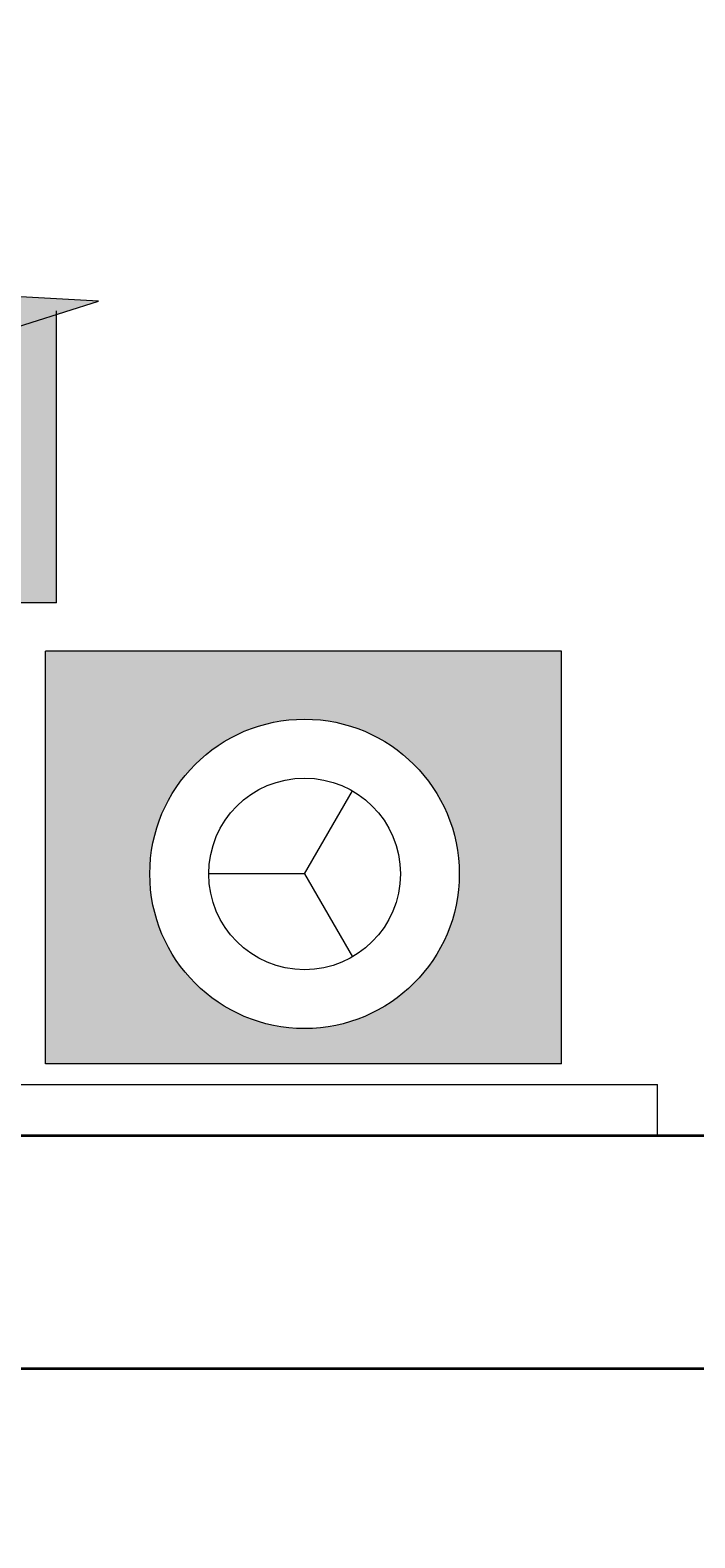
# Model space of a CAD drawing. Units: millimetres. Extents: x 27017497 to 27018854, y 7058029 to 7059154.
# Tile 76 of 91: x 27018436 to 27018462, y 7058126 to 7058185. Entities that reach past the tile are written whole.
import ezdxf

# ---------------------------------------------------------------- set-up
doc = ezdxf.new("R2010")
doc.units = ezdxf.units.MM
for name, color, linetype, lineweight in [('A-ANNO-DIMS', 2, 'Continuous', 18), ('A-FURN', 8, 'Continuous', 18), ('A-WALL', 7, 'Continuous', 35)]:
    doc.layers.add(name, color=color, linetype=linetype, lineweight=lineweight)
doc.layers.add('A-FURN-PATT', color=177, linetype='Continuous', lineweight=13, true_color=0x293189)
doc.styles.get("Standard").update_dxf_attribs({"font": 'arial.ttf'})
doc.dimstyles.get("Standard").update_dxf_attribs({"dimtxt": 0.18, "dimasz": 0.18, "dimexe": 0.18, "dimexo": 0.0625, "dimgap": 0.09, "dimtad": 0, "dimtih": 1, "dimtoh": 1, "dimdec": 4, "dimzin": 0, "dimdsep": 46, "dimtxsty": 'Standard', "dimcen": 0.09, "dimadec": 0, "dimazin": 0, "dimtfac": 1, "dimtdec": 4, "dimtofl": 0, "dimtmove": 0, "dimatfit": 3, "dimfxl": 1, "dimtolj": 1, "dimtzin": 0, "dimarcsym": 0})

# ---------------------------------------------------------------- blocks, each defined once
blk = doc.blocks.new('CAMMAT')
for p, q in [((1.2731, 0), (-1.2731, 0)), ((-1.2731, 0), (-1.2731, -0.05)), ((1.2731, -0.05), (-1.2731, -0.05)), ((-1.18, -0.07), (-1.18, -0.47)), ((-1.18, -0.07), (-0.68, -0.07)), ((-0.68, -0.07), (-0.68, -0.47)), ((-0.931, -0.2541), (-0.9775, -0.1737)), ((-0.931, -0.2541), (-0.9775, -0.3346)), ((-0.931, -0.2541), (-0.8381, -0.2541)), ((-1.18, -0.47), (-0.68, -0.47)), ((-0.6904, -0.5169), (-0.6904, -0.8)), ((-0.6904, -0.5169), (0.6826, -0.5169)), ((0.0535, -0.5623), (-0.7312, -0.8093))]:
    blk.add_line(p, q)
blk.add_lwpolyline([(-0.7312, -0.8093), (-0.5683, -0.8185), (-0.4451, -0.828), (-0.3552, -0.8406), (-0.2919, -0.8591), (-0.2489, -0.8862), (-0.2196, -0.9248), (-0.1975, -0.9777), (-0.1761, -1.0476)])
for radius in [0.15, 0.0929]:
    blk.add_circle((-0.931, -0.2541), radius)
blk = doc.blocks.new('*D47')
at = {"layer": 'A-ANNO-DIMS', "color": 0, "lineweight": -2, "transparency": 16777216}
for p, q in [((27017561.166, 7058294.35), (27017561.166, 7058028.6)), ((27018790.606, 7058294.35), (27018790.606, 7058028.6)), ((27017561.346, 7058028.78), (27018175.431, 7058028.78)), ((27018790.426, 7058028.78), (27018176.341, 7058028.78))]:
    blk.add_line(p, q, dxfattribs=at)
at = {"layer": 'A-ANNO-DIMS', "color": 0, "transparency": 16777216}
for points in [[(27017561.346, 7058028.81), (27017561.346, 7058028.75), (27017561.166, 7058028.78)], [(27018790.426, 7058028.81), (27018790.426, 7058028.75), (27018790.606, 7058028.78)]]:
    blk.add_solid(points, dxfattribs=at)
at = {"layer": 'Defpoints', "color": 0, "transparency": 16777216}
for p in [(27017561.166, 7058294.412), (27018790.606, 7058294.412), (27018790.606, 7058028.78)]:
    blk.add_point(p, dxfattribs=at)
at = {"layer": 'A-ANNO-DIMS', "color": 0, "transparency": 16777216, "insert": (27018175.886, 7058028.78), "char_height": 0.18, "attachment_point": 5}
blk.add_mtext('\\A1;1229.4', dxfattribs=at)
blk = doc.blocks.new('*D48')
at = {"layer": 'A-ANNO-DIMS', "color": 0, "lineweight": -2, "transparency": 16777216}
for p, q in [((27018463.498, 7058622.912), (27017497.536, 7058622.912)), ((27017497.716, 7058622.732), (27017497.716, 7058357.753)), ((27017497.716, 7058092.41), (27017497.716, 7058357.389)), ((27018555.129, 7058092.23), (27017497.536, 7058092.23))]:
    blk.add_line(p, q, dxfattribs=at)
at = {"layer": 'A-ANNO-DIMS', "color": 0, "transparency": 16777216}
for points in [[(27017497.686, 7058622.732), (27017497.746, 7058622.732), (27017497.716, 7058622.912)], [(27017497.686, 7058092.41), (27017497.746, 7058092.41), (27017497.716, 7058092.23)]]:
    blk.add_solid(points, dxfattribs=at)
at = {"layer": 'Defpoints', "color": 0, "transparency": 16777216}
for p in [(27018463.561, 7058622.912), (27017497.716, 7058092.23), (27018555.192, 7058092.23)]:
    blk.add_point(p, dxfattribs=at)
at = {"layer": 'A-ANNO-DIMS', "color": 0, "transparency": 16777216, "insert": (27017497.716, 7058357.571), "char_height": 0.18, "attachment_point": 5}
blk.add_mtext('\\A1;530.7', dxfattribs=at)

msp = doc.modelspace()

# ---------------------------------------------------------------- hatches: boundary and pattern name
at = {"layer": 'A-FURN-PATT'}
h = msp.add_hatch(color=256, dxfattribs=at)
h.dxf.hatch_style = 1
h.paths.add_polyline_path([(27018435.86, 7058218.784, 0.414214), (27018434.267, 7058220.377), (27018385.674, 7058220.377, 0.414214), (27018384.081, 7058218.784), (27018384.081, 7058174.59), (27018387.977, 7058174.891), (27018391.56, 7058175.393), (27018394.078, 7058176.128), (27018395.791, 7058177.21), (27018396.958, 7058178.748), (27018397.838, 7058180.854), (27018398.69, 7058183.639), (27018399.293, 7058180.835), (27018399.836, 7058178.594), (27018400.426, 7058176.691), (27018401.17, 7058174.899), (27018402.177, 7058172.991), (27018403.552, 7058170.741), (27018405.403, 7058167.922), (27018407.838, 7058164.308), (27018410.273, 7058167.922), (27018412.124, 7058170.741), (27018413.499, 7058172.991), (27018414.506, 7058174.899), (27018415.25, 7058176.691), (27018415.84, 7058178.594), (27018416.383, 7058180.835), (27018416.986, 7058183.639), (27018417.838, 7058180.854), (27018418.718, 7058178.748), (27018419.885, 7058177.21), (27018421.598, 7058176.128), (27018424.116, 7058175.393), (27018427.699, 7058174.891), (27018432.604, 7058174.513), (27018435.86, 7058174.329)])
h.paths.add_polyline_path([(27018439.093, 7058174.146), (27018432.604, 7058174.513), (27018427.699, 7058174.891), (27018424.116, 7058175.393), (27018421.598, 7058176.128), (27018419.885, 7058177.21), (27018418.718, 7058178.748), (27018417.838, 7058180.854), (27018416.986, 7058183.639), (27018416.383, 7058180.835), (27018415.84, 7058178.594), (27018415.25, 7058176.691), (27018414.506, 7058174.899), (27018413.499, 7058172.991), (27018412.124, 7058170.741), (27018410.273, 7058167.922), (27018407.838, 7058164.308)])
h.paths.add_polyline_path([(27018403.552, 7058170.741), (27018402.177, 7058172.991), (27018401.17, 7058174.899), (27018400.426, 7058176.691), (27018399.836, 7058178.594), (27018399.293, 7058180.835), (27018398.69, 7058183.639), (27018397.838, 7058180.854), (27018396.958, 7058178.748), (27018395.791, 7058177.21), (27018394.078, 7058176.128), (27018391.56, 7058175.393), (27018387.977, 7058174.891), (27018383.071, 7058174.513), (27018376.583, 7058174.146), (27018407.838, 7058164.308), (27018405.403, 7058167.922)])
h.paths.add_polyline_path([(27018437.469, 7058173.635), (27018407.838, 7058164.308), (27018382.784, 7058172.194), (27018382.784, 7058162.502), (27018437.469, 7058162.502)])
h.paths.add_polyline_path([(27018435.86, 7058162.502), (27018384.081, 7058162.502), (27018384.081, 7058146.294, 0.414214), (27018385.674, 7058144.7), (27018434.267, 7058144.7, 0.414214), (27018435.86, 7058146.294)])
h.paths.add_polyline_path([(27018407.684, 7058159.418, -0.41419), (27018408.879, 7058158.223), (27018408.879, 7058148.664, -0.414237), (27018407.684, 7058147.469), (27018386.224, 7058147.469, -0.41419), (27018385.029, 7058148.663), (27018385.029, 7058158.223, -0.414237), (27018386.224, 7058159.418)], flags=16)
h.paths.add_polyline_path([(27018411.821, 7058159.418), (27018433.28, 7058159.418, -0.41419), (27018434.475, 7058158.223), (27018434.475, 7058148.664, -0.414237), (27018433.28, 7058147.469), (27018411.821, 7058147.469, -0.414214), (27018410.626, 7058148.664), (27018410.626, 7058158.223, -0.414214)], flags=16)
h.paths.add_polyline_path([(27018382.886, 7058160.632), (27018362.971, 7058160.632), (27018362.971, 7058144.7), (27018382.886, 7058144.7)])
h.paths.add_polyline_path([(27018379.136, 7058152.033, -1), (27018367.187, 7058152.033, -1)], flags=16)
h.paths.add_polyline_path([(27018376.861, 7058152.033, -1), (27018369.461, 7058152.033, -1)], flags=0)
h.paths.add_polyline_path([(27018456.97, 7058160.632), (27018437.055, 7058160.632), (27018437.055, 7058144.7), (27018456.97, 7058144.7)])
h.paths.add_polyline_path([(27018453.028, 7058152.033, -1), (27018441.079, 7058152.033, -1)], flags=16)
h.paths.add_polyline_path([(27018450.754, 7058152.033, -1), (27018443.354, 7058152.033, -1)], flags=0)
h.paths.add_polyline_path([(27018434.475, 7058158.223, 0.41419), (27018433.28, 7058159.418), (27018411.821, 7058159.418, 0.414214), (27018410.626, 7058158.223), (27018410.626, 7058148.664, 0.414214), (27018411.821, 7058147.469), (27018433.28, 7058147.469, 0.414237), (27018434.475, 7058148.664)], flags=0)

# ---------------------------------------------------------------- linework, layer by layer
at = {"layer": 'A-WALL'}
for p, q in [((27018468.106, 7058141.912), (27018319.606, 7058141.912)), ((27018468.106, 7058132.912), (27018310.606, 7058132.912))]:
    msp.add_line(p, q, dxfattribs=at)

# ---------------------------------------------------------------- block references
at = {"layer": 'A-FURN', "xscale": 39.82996475819422, "yscale": 39.82996475819422, "zscale": 39.82996475819422, "rotation": 180}
msp.add_blockref('CAMMAT', (27018409.97, 7058141.912), dxfattribs=at)

# ---------------------------------------------------------------- dimensions: what is measured, and where the dimension line sits
at = {"layer": 'A-ANNO-DIMS'}
dim = msp.add_linear_dim(base=(27017497.716, 7058092.23), p1=(27018463.561, 7058622.912), p2=(27018555.192, 7058092.23), angle=90, dimstyle='Standard', override={"dimdec": 1, "dimlfac": 1, "dimrnd": 0, "dimzin": 0, "dimdsep": 46, "dimlunit": 2}, dxfattribs=at)
dim.commit()
dim.dimension.update_dxf_attribs({"geometry": '*D48', "text_midpoint": (27017497.716, 7058357.571)})
dim = msp.add_linear_dim(base=(27018790.606, 7058028.78), p1=(27017561.166, 7058294.412), p2=(27018790.606, 7058294.412), dimstyle='Standard', override={"dimdec": 1, "dimlfac": 1, "dimrnd": 0, "dimzin": 0, "dimdsep": 46, "dimlunit": 2}, dxfattribs=at)
dim.commit()
dim.dimension.update_dxf_attribs({"geometry": '*D47', "text_midpoint": (27018175.886, 7058028.78)})

doc.saveas('drawing.dxf')
